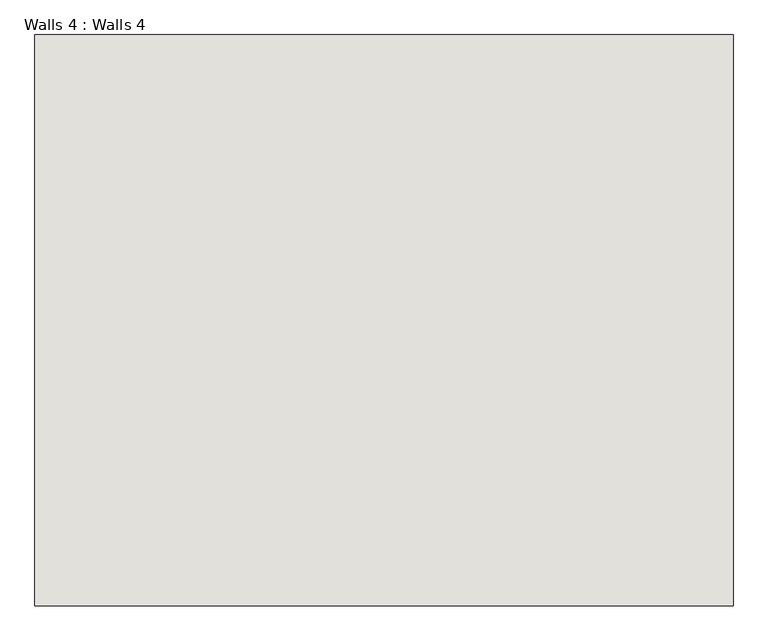
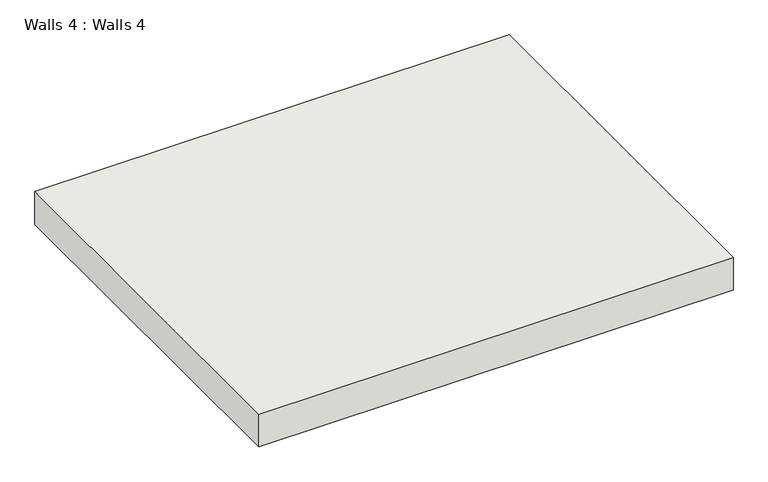
"""IFC4 building model written with IfcOpenShell, lengths in millimetres: wall geometry, Walls 4 : Walls 4."""

from ifc_helpers import new_model, si_unit, frame, origin, place, context, project, spatial, polyline, outline, extrude, source, transform, mapped, element, save


def walls_4_walls_4_c70d8470(model_context):
    return source(origin(), model_context, "Body", "SweptSolid", [
        extrude(outline(polyline([(545.5980639, 709.3437087), (545.5980639, -7318.3201523), (-9260.4019361, -7318.3201523), (-9260.4019361, 709.3437087), (545.5980639, 709.3437087)])), frame((0.0, 0.0, 2327.8881187), z_axis=(0.0, 0.0, 1.0), x_axis=(1.0, 0.0, 0.0)), (0.0, 0.0, 1.0), 720.1118813),
    ])


if __name__ == "__main__":
    model = new_model("IFC4")
    model_context = context("Model", 3, world=origin())
    ifc_project = project(units=[si_unit("LENGTHUNIT", "METRE", prefix="MILLI")], contexts=[model_context])
    site = spatial("IfcSite", under=ifc_project)
    building = spatial("IfcBuilding", under=site)
    placement = place(None, origin())
    walls_4_walls_4_shape = walls_4_walls_4_c70d8470(model_context)
    element("IfcWall", 1, ObjectType="Walls 4 : Walls 4", at=placement, inside=building, context=model_context, shape_type="MappedRepresentation", body=[
        mapped(walls_4_walls_4_shape, transform((0.0, 0.0, 0.0), x_axis=(1.0, 0.0, 0.0), y_axis=(0.0, 1.0, 0.0), z_axis=(0.0, 0.0, 1.0))),
    ])
    save(model, "model.ifc")

# Revit data of these elements
# Element 1 (IfcWall, "Walls 4 : Walls 4")
#   Materials on its faces: "Default Wall"
# Materials
#   "Default Wall": colour RGB 80 80 80, transparency 0
